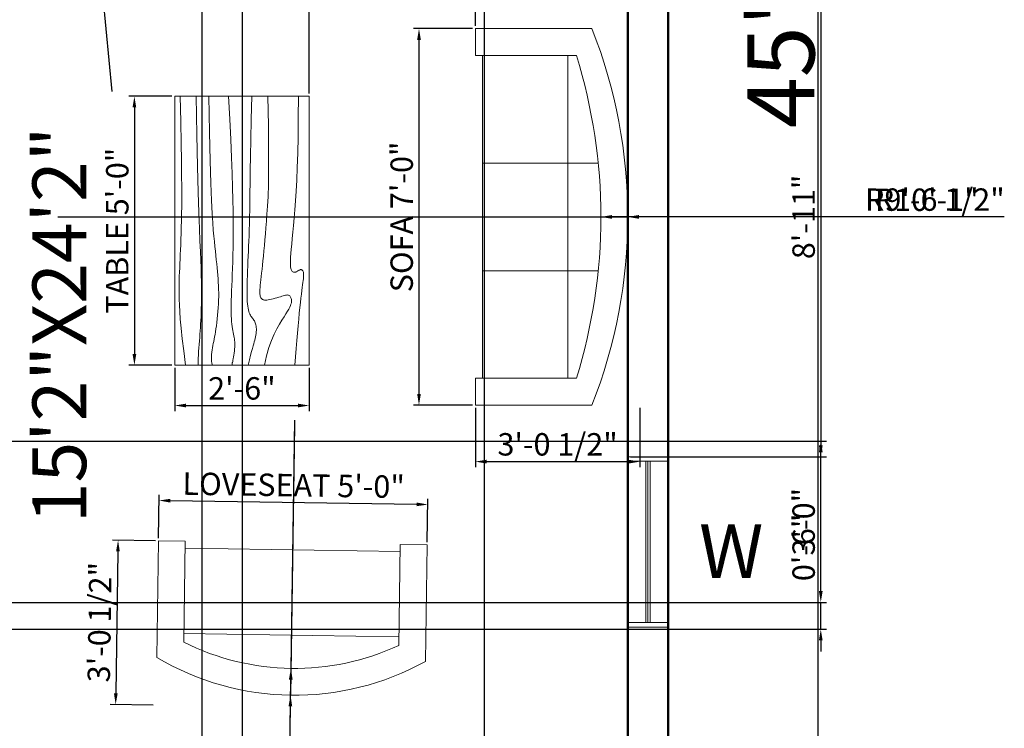
# Model space of a CAD drawing. Units: inches. Extents: x 2050 to 2529, y 1266 to 1968.
# Tile 3 of 5: x 2310 to 2529, y 1427 to 1585. Entities that reach past the tile are written whole.
import ezdxf

# ---------------------------------------------------------------- set-up
doc = ezdxf.new("R2010")
doc.units = ezdxf.units.IN
for name, color, linetype, lineweight in [('A-ANNO-DIMS', 2, 'Continuous', 18), ('A-ANNO-TEXT', 7, 'Continuous', 18), ('A-AREA-IDEN', 7, 'Continuous', 25), ('A-FURN', 8, 'Continuous', 18), ('A-GLAZ', 4, 'Continuous', 18), ('A-WALL', 7, 'Continuous', 50)]:
    doc.layers.add(name, color=color, linetype=linetype, lineweight=lineweight)
doc.styles.get("Standard").update_dxf_attribs({"font": 'arial.ttf'})
doc.dimstyles.new('ISO-25', dxfattribs={"dimtxt": 5, "dimasz": 2.5, "dimexe": 1.25, "dimexo": 0.625, "dimtad": 1, "dimlunit": 3, "dimtxsty": 'Standard', "dimcen": 2.5, "dimadec": 0, "dimazin": 0, "dimtfac": 1, "dimtmove": 0, "dimatfit": 3, "dimfxl": 1, "dimarcsym": 0})

# ---------------------------------------------------------------- blocks, each defined once
blk = doc.blocks.new('*D2')
at = {"layer": 'A-ANNO-DIMS', "color": 0, "lineweight": -2, "transparency": 16777216}
for p, q in [((2454.92, 1844.72), (2488.97, 1844.72)), ((2487.72, 1842.22), (2487.72, 1307.22)), ((2454.92, 1304.72), (2488.97, 1304.72))]:
    blk.add_line(p, q, dxfattribs=at)
at = {"layer": 'A-ANNO-DIMS', "color": 0, "transparency": 16777216}
for points in [[(2487.3, 1842.22), (2488.13, 1842.22), (2487.72, 1844.72)], [(2487.3, 1307.22), (2488.13, 1307.22), (2487.72, 1304.72)]]:
    blk.add_solid(points, dxfattribs=at)
at = {"layer": 'Defpoints', "color": 0, "transparency": 16777216}
for p in [(2454.29, 1844.72), (2454.29, 1304.72), (2487.72, 1304.72)]:
    blk.add_point(p, dxfattribs=at)
at = {"layer": 'A-ANNO-DIMS', "color": 0, "transparency": 16777216, "insert": (2479.46, 1574.72), "char_height": 5, "attachment_point": 5, "rotation": 90}
blk.add_mtext("{\\H3x;45'}", dxfattribs=at)
blk = doc.blocks.new('Table - Rectangular Woodgrain 60 x 30 in.')
for p, q in [((0, 0), (0, -30)), ((60, 0), (0, 0)), ((60, -30), (60, 0)), ((0, -30), (60, -30))]:
    blk.add_line(p, q)
for points in [[(0, -2.4), (4.8155, -2.418), (9.0302, -2.4688), (12.709, -2.5477), (15.9167, -2.65), (18.7181, -2.7711), (21.1781, -2.9063), (23.3616, -3.0508), (25.3333, -3.2), (27.1477, -3.3495), (28.8172, -3.4958), (30.3437, -3.636), (31.7291, -3.7667), (32.9756, -3.8849), (34.0849, -3.9875), (35.059, -4.0714), (35.9, -4.1334), (36.6114, -4.1711), (37.2041, -4.1854), (37.6906, -4.1779), (38.0833, -4.15), (38.3948, -4.1034), (38.6375, -4.0396), (38.8239, -3.9602), (38.9666, -3.8667), (39.0764, -3.7608), (39.1573, -3.6448), (39.2116, -3.521), (39.2416, -3.3917), (39.2498, -3.2593), (39.2385, -3.1261), (39.21, -2.9944), (39.1666, -2.8667), (39.111, -2.7447), (39.0468, -2.6281), (38.978, -2.5163), (38.9083, -2.4083), (38.8418, -2.3035), (38.7823, -2.201), (38.7337, -2.1001), (38.7, -2), (38.6844, -1.9003), (38.6875, -1.8021), (38.7094, -1.707), (38.75, -1.6167), (38.8094, -1.5326), (38.8875, -1.4563), (38.9844, -1.3893), (39.1, -1.3333), (39.2351, -1.2896), (39.3937, -1.2583), (39.5804, -1.2396), (39.8, -1.2333), (40.057, -1.2396), (40.3562, -1.2583), (40.7023, -1.2896), (41.1, -1.3333), (41.5547, -1.3895), (42.0755, -1.4573), (42.6721, -1.5361), (43.3542, -1.625), (44.1316, -1.7233), (45.014, -1.8302), (46.0114, -1.9449), (47.1333, -2.0667), (48.3862, -2.1947), (49.7625, -2.3281), (51.2513, -2.4663), (52.8416, -2.6083), (54.5226, -2.7535), (56.2833, -2.9011), (58.1127, -3.0501), (60, -3.2)], [(0, -9.2), (6.5759, -9.0858), (11.9385, -9.0365), (16.2527, -9.0418), (19.6833, -9.0917), (22.3952, -9.1759), (24.5531, -9.2844), (26.322, -9.4069), (27.8666, -9.5333), (29.3241, -9.6553), (30.7203, -9.7719), (32.0532, -9.8837), (33.3208, -9.9917), (34.5213, -10.0965), (35.6526, -10.199), (36.7128, -10.2999), (37.7, -10.4), (38.6129, -10.4996), (39.4531, -10.5969), (40.223, -10.6895), (40.925, -10.775), (41.5613, -10.8512), (42.1344, -10.9156), (42.6465, -10.966), (43.1, -11), (43.4976, -11.0158), (43.8437, -11.0136), (44.143, -10.9942), (44.4, -10.9583), (44.6195, -10.9069), (44.8062, -10.8406), (44.9648, -10.7603), (45.1, -10.6667), (45.2155, -10.5598), (45.3114, -10.4365), (45.3871, -10.2929), (45.4416, -10.125), (45.4743, -9.929), (45.4844, -9.7011), (45.4709, -9.4371), (45.4333, -9.1333), (45.3716, -8.7883), (45.2896, -8.4104), (45.1919, -8.0107), (45.0833, -7.6), (44.9685, -7.1893), (44.8521, -6.7896), (44.7388, -6.4117), (44.6333, -6.0667), (44.54, -5.7628), (44.4614, -5.4979), (44.4001, -5.2675), (44.3583, -5.0667), (44.3384, -4.8909), (44.3427, -4.7354), (44.3736, -4.5956), (44.4333, -4.4667), (44.5236, -4.3453), (44.6427, -4.2333), (44.7884, -4.1339), (44.9583, -4.05), (45.1501, -3.9849), (45.3614, -3.9417), (45.59, -3.9234), (45.8333, -3.9333), (46.0915, -3.9749), (46.3734, -4.0531), (46.6906, -4.1736), (47.0542, -4.3417), (47.4756, -4.5629), (47.9661, -4.8427), (48.5372, -5.1866), (49.2, -5.6), (49.9676, -6.0844), (50.8594, -6.625), (51.8965, -7.2031), (53.1, -7.8), (54.491, -8.3969), (56.0906, -8.975), (57.9199, -9.5156), (60, -10)], [(0, -12.8), (5.1847, -12.9322), (9.6213, -13.0323), (13.3963, -13.1059), (16.5958, -13.1583), (19.3063, -13.1952), (21.614, -13.2219), (23.6054, -13.2439), (25.3666, -13.2667), (26.9728, -13.2947), (28.4531, -13.3281), (29.8256, -13.3663), (31.1083, -13.4083), (32.3191, -13.4535), (33.476, -13.501), (34.597, -13.5501), (35.7, -13.6), (36.7984, -13.6497), (37.8875, -13.6979), (38.9578, -13.743), (40, -13.7833), (41.0047, -13.8174), (41.9625, -13.8438), (42.864, -13.8607), (43.7, -13.8667), (44.4631, -13.8604), (45.1552, -13.8417), (45.7801, -13.8104), (46.3416, -13.7667), (46.8439, -13.7104), (47.2906, -13.6417), (47.6858, -13.5604), (48.0333, -13.4667), (48.3375, -13.3608), (48.6042, -13.2448), (48.8396, -13.121), (49.05, -12.9917), (49.2417, -12.8593), (49.4208, -12.7261), (49.5937, -12.5944), (49.7667, -12.4667), (49.9452, -12.3451), (50.1323, -12.2313), (50.3303, -12.1268), (50.5416, -12.0333), (50.7686, -11.9524), (51.0135, -11.8854), (51.2788, -11.8341), (51.5666, -11.8), (51.8785, -11.7843), (52.2116, -11.7865), (52.562, -11.8059), (52.926, -11.8417), (53.2998, -11.8931), (53.6795, -11.9594), (54.0614, -12.0397), (54.4416, -12.1333), (54.8223, -12.2401), (55.2293, -12.3625), (55.6942, -12.5037), (56.2489, -12.6667), (56.9251, -12.8547), (57.7545, -13.0708), (58.7689, -13.3182), (60, -13.6)], [(0, -18), (5.124, -17.7273), (9.6609, -17.5057), (13.6705, -17.3303), (17.2125, -17.1958), (20.3467, -17.0973), (23.1328, -17.0297), (25.6307, -16.9878), (27.9, -16.9667), (29.9928, -16.9617), (31.9302, -16.9703), (33.7254, -16.9907), (35.3917, -17.0208), (36.9423, -17.0588), (38.3906, -17.1026), (39.7499, -17.1503), (41.0333, -17.2), (42.2519, -17.2496), (43.4073, -17.2969), (44.4986, -17.3395), (45.525, -17.375), (46.4858, -17.4012), (47.3802, -17.4156), (48.2074, -17.416), (48.9667, -17.4), (49.6583, -17.3662), (50.2872, -17.3167), (50.8595, -17.2547), (51.3812, -17.1833), (51.8584, -17.1057), (52.2971, -17.025), (52.7034, -16.9443), (53.0833, -16.8667), (53.443, -16.7951), (53.789, -16.7313), (54.128, -16.6768), (54.4666, -16.6334), (54.8115, -16.6024), (55.1693, -16.5854), (55.5465, -16.5841), (55.95, -16.6), (56.3828, -16.6337), (56.8346, -16.6823), (57.2915, -16.7418), (57.7396, -16.8084), (58.165, -16.878), (58.5539, -16.9469), (58.8924, -17.0111), (59.1666, -17.0667), (59.3679, -17.1107), (59.5078, -17.1438), (59.6032, -17.1675), (59.6708, -17.1833), (59.7275, -17.193), (59.7901, -17.1979), (59.8753, -17.1998), (60, -17.2)], [(0, -22.4), (8.0098, -22.2501), (14.4094, -22.1011), (19.4168, -21.9535), (23.25, -21.8083), (26.1269, -21.6663), (28.2656, -21.5281), (29.884, -21.3947), (31.2, -21.2667), (32.3967, -21.1448), (33.5172, -21.0292), (34.5697, -20.9198), (35.5625, -20.8167), (36.5037, -20.7198), (37.4015, -20.6292), (38.2642, -20.5448), (39.1, -20.4667), (39.9164, -20.3951), (40.7187, -20.3313), (41.5117, -20.2768), (42.3, -20.2333), (43.0883, -20.2024), (43.8812, -20.1854), (44.6836, -20.1841), (45.5, -20.2), (46.3328, -20.234), (47.1747, -20.2844), (48.0163, -20.3488), (48.8479, -20.425), (49.66, -20.5106), (50.4429, -20.6031), (51.1872, -20.7004), (51.8833, -20.8), (52.5246, -20.8999), (53.1166, -20.9995), (53.6681, -21.0983), (54.1875, -21.1958), (54.6834, -21.2919), (55.1646, -21.3859), (55.6394, -21.4777), (56.1167, -21.5667), (56.6028, -21.6515), (57.0961, -21.7266), (57.5929, -21.7852), (58.0896, -21.8208), (58.5823, -21.8268), (59.0674, -21.7964), (59.5412, -21.723), (60, -21.6)], [(0, -25.2), (8.6355, -25.0504), (15.7026, -24.9031), (21.4049, -24.7606), (25.9458, -24.625), (29.529, -24.4988), (32.3578, -24.3844), (34.6359, -24.284), (36.5667, -24.2), (38.3213, -24.1341), (39.9417, -24.0854), (41.437, -24.0523), (42.8167, -24.0333), (44.0901, -24.0268), (45.2667, -24.0313), (46.3557, -24.0451), (47.3667, -24.0667), (48.309, -24.0947), (49.1928, -24.1287), (50.0284, -24.168), (50.826, -24.2125), (51.5959, -24.2617), (52.3483, -24.3151), (53.0935, -24.3725), (53.8417, -24.4334), (54.6009, -24.497), (55.3699, -24.561), (56.1454, -24.6226), (56.9239, -24.6792), (57.7021, -24.7279), (58.4764, -24.7662), (59.2435, -24.7911), (60, -24.8)], [(0, -28.8), (5.6867, -28.6681), (10.45, -28.5698), (14.407, -28.5012), (17.675, -28.4584), (20.3711, -28.4374), (22.6125, -28.4344), (24.5164, -28.4455), (26.2, -28.4667), (27.762, -28.4947), (29.2276, -28.5281), (30.6033, -28.5663), (31.8958, -28.6084), (33.1118, -28.6535), (34.2578, -28.7011), (35.3405, -28.7501), (36.3666, -28.8), (37.3443, -28.8497), (38.288, -28.8974), (39.2137, -28.9412), (40.1375, -28.9792), (41.0753, -29.0093), (42.0432, -29.0297), (43.0572, -29.0384), (44.1333, -29.0333), (45.2936, -29.0114), (46.5843, -28.9641), (48.0579, -28.8816), (49.7666, -28.7542), (51.7629, -28.5721), (54.0989, -28.3255), (56.8272, -28.0048), (60, -27.6)]]:
    blk.add_lwpolyline(points)
blk = doc.blocks.new('Sofa - Roundback 7 ft.')
for p, q in [((-12.00002, -32.4421), (-12.00003, -6.5971)), ((11.99997, -32.4421), (11.99998, -6.5971)), ((-36.000027, -34), (-36.000027, -11.4696)), ((35.99998, -34), (35.99998, -11.4696)), ((-35.999844, -13.3819), (35.9998, -13.3819)), ((-36.000027, -32.4421), (35.99998, -32.4421))]:
    blk.add_line(p, q)
for points in [[(-36.000027, -34), (-42.000027, -34), (-42.000027, -8)], [(41.99998, -8), (41.99998, -34), (35.99998, -34)]]:
    blk.add_lwpolyline(points)
for centre, radius, start, end in [((0, -114.25), 114.25, 68.43141, 111.5686), ((-0.00001, -127.1968), 121.1968, 72.72033, 107.2797)]:
    blk.add_arc(centre, radius, start, end)
blk = doc.blocks.new('Sofa - Roundback Loveseat 5 ft.')
for p, q in [((0, -32.44198), (0, -5.99998)), ((-24, -33.99998), (-24, -11.46958)), ((24.00004, -33.99998), (24.00004, -11.46958)), ((-23.9998, -13.38178), (23.99986, -13.38178)), ((-24, -32.44198), (24.00004, -32.44198))]:
    blk.add_line(p, q)
for points in [[(-24, -33.99998), (-30, -33.99998), (-30, -7.99998)], [(30.00004, -7.99998), (30.00004, -33.99998), (24.00004, -33.99998)]]:
    blk.add_lwpolyline(points)
for centre, radius, start, end in [((0, -60.24998), 60.24998, 60.13715, 119.8628), ((0, -61.38438), 55.38444, 64.32083, 115.6792)]:
    blk.add_arc(centre, radius, start, end)
blk = doc.blocks.new('WIN-36IN')
for p, q in [((0, 9), (0, 0)), ((1, 9), (1, 0)), ((37, 9), (37, 0)), ((38, 9), (38, 0)), ((1, 5), (37, 5)), ((1, 4.5), (37, 4.5)), ((1, 4), (37, 4))]:
    blk.add_line(p, q)
blk = doc.blocks.new('*D32')
at = {"layer": 'A-ANNO-DIMS', "color": 0, "lineweight": -2, "transparency": 16777216}
for p, q in [((2343.55, 1567.64), (2333.92, 1567.64)), ((2335.17, 1565.14), (2335.17, 1510.14)), ((2343.55, 1507.64), (2333.92, 1507.64))]:
    blk.add_line(p, q, dxfattribs=at)
at = {"layer": 'A-ANNO-DIMS', "color": 0, "transparency": 16777216}
for points in [[(2334.76, 1565.14), (2335.59, 1565.14), (2335.17, 1567.64)], [(2334.76, 1510.14), (2335.59, 1510.14), (2335.17, 1507.64)]]:
    blk.add_solid(points, dxfattribs=at)
at = {"layer": 'Defpoints', "color": 0, "transparency": 16777216}
for p in [(2344.17, 1567.64), (2335.17, 1507.64), (2344.17, 1507.64)]:
    blk.add_point(p, dxfattribs=at)
at = {"layer": 'A-ANNO-DIMS', "color": 0, "transparency": 16777216, "insert": (2332, 1537.64), "char_height": 5, "attachment_point": 5, "rotation": 90}
blk.add_mtext('TABLE 5\'-0"', dxfattribs=at)
blk = doc.blocks.new('*D33')
at = {"layer": 'A-ANNO-DIMS', "color": 0, "lineweight": -2, "transparency": 16777216}
for p, q in [((2344.17, 1507.01), (2344.17, 1497.39)), ((2374.17, 1507.01), (2374.17, 1497.39)), ((2346.67, 1498.64), (2371.67, 1498.64))]:
    blk.add_line(p, q, dxfattribs=at)
at = {"layer": 'A-ANNO-DIMS', "color": 0, "transparency": 16777216}
for points in [[(2346.67, 1499.05), (2346.67, 1498.22), (2344.17, 1498.64)], [(2371.67, 1499.05), (2371.67, 1498.22), (2374.17, 1498.64)]]:
    blk.add_solid(points, dxfattribs=at)
at = {"layer": 'Defpoints', "color": 0, "transparency": 16777216}
for p in [(2344.17, 1507.64), (2374.17, 1507.64), (2374.17, 1498.64)]:
    blk.add_point(p, dxfattribs=at)
at = {"layer": 'A-ANNO-DIMS', "color": 0, "transparency": 16777216, "insert": (2359.17, 1501.81), "char_height": 5, "attachment_point": 5}
blk.add_mtext('2\'-6"', dxfattribs=at)
blk = doc.blocks.new('*D38')
at = {"layer": 'A-ANNO-DIMS', "color": 0, "lineweight": -2, "transparency": 16777216}
for p, q in [((2410.67, 1582.72), (2397.44, 1582.72)), ((2398.69, 1580.22), (2398.69, 1501.22)), ((2410.67, 1498.72), (2397.44, 1498.72))]:
    blk.add_line(p, q, dxfattribs=at)
at = {"layer": 'A-ANNO-DIMS', "color": 0, "transparency": 16777216}
for points in [[(2398.28, 1580.22), (2399.11, 1580.22), (2398.69, 1582.72)], [(2398.28, 1501.22), (2399.11, 1501.22), (2398.69, 1498.72)]]:
    blk.add_solid(points, dxfattribs=at)
at = {"layer": 'Defpoints', "color": 0, "transparency": 16777216}
for p in [(2411.29, 1582.72), (2398.69, 1498.72), (2411.29, 1498.72)]:
    blk.add_point(p, dxfattribs=at)
at = {"layer": 'A-ANNO-DIMS', "color": 0, "transparency": 16777216, "insert": (2395.48, 1540.72), "char_height": 5, "attachment_point": 5, "rotation": 90}
blk.add_mtext('SOFA 7\'-0"', dxfattribs=at)
blk = doc.blocks.new('*D39')
at = {"layer": 'A-ANNO-DIMS', "color": 0, "lineweight": -2, "transparency": 16777216}
for p, q in [((2411.29, 1498.1), (2411.29, 1484.87)), ((2447.96, 1498.1), (2447.96, 1484.87)), ((2413.79, 1486.12), (2445.46, 1486.12))]:
    blk.add_line(p, q, dxfattribs=at)
at = {"layer": 'A-ANNO-DIMS', "color": 0, "transparency": 16777216}
for points in [[(2413.79, 1486.54), (2413.79, 1485.7), (2411.29, 1486.12)], [(2445.46, 1486.54), (2445.46, 1485.7), (2447.96, 1486.12)]]:
    blk.add_solid(points, dxfattribs=at)
at = {"layer": 'Defpoints', "color": 0, "transparency": 16777216}
for p in [(2411.29, 1498.72), (2447.96, 1498.72), (2447.96, 1486.12)]:
    blk.add_point(p, dxfattribs=at)
at = {"layer": 'A-ANNO-DIMS', "color": 0, "transparency": 16777216, "insert": (2429.63, 1489.33), "char_height": 5, "attachment_point": 5}
blk.add_mtext('3\'-0 1/2"', dxfattribs=at)
blk = doc.blocks.new('*D40')
at = {"layer": 'A-ANNO-DIMS', "color": 0, "lineweight": -2, "transparency": 16777216}
for p, q in [((2340.54, 1469.07), (2340.68, 1478.69)), ((2398.16, 1476.58), (2343.17, 1477.4)), ((2400.54, 1468.17), (2400.68, 1477.8))]:
    blk.add_line(p, q, dxfattribs=at)
at = {"layer": 'A-ANNO-DIMS', "color": 0, "transparency": 16777216}
for points in [[(2343.17, 1477.82), (2343.16, 1476.99), (2340.67, 1477.44)], [(2398.17, 1477), (2398.15, 1476.17), (2400.66, 1476.55)]]:
    blk.add_solid(points, dxfattribs=at)
at = {"layer": 'Defpoints', "color": 0, "transparency": 16777216}
for p in [(2340.67, 1477.44), (2340.53, 1468.44), (2400.53, 1467.55)]:
    blk.add_point(p, dxfattribs=at)
at = {"layer": 'A-ANNO-DIMS', "color": 0, "transparency": 16777216, "insert": (2370.71, 1480.21), "char_height": 5, "attachment_point": 5, "rotation": 359.1468}
blk.add_mtext('LOVESEAT 5\'-0"', dxfattribs=at)
blk = doc.blocks.new('*D41')
at = {"layer": 'A-ANNO-DIMS', "color": 0, "lineweight": -2, "transparency": 16777216}
for p, q in [((2339.91, 1468.45), (2330.28, 1468.59)), ((2331.5, 1466.08), (2331.02, 1434.41)), ((2339.36, 1431.79), (2329.74, 1431.93))]:
    blk.add_line(p, q, dxfattribs=at)
at = {"layer": 'A-ANNO-DIMS', "color": 0, "transparency": 16777216}
for points in [[(2331.08, 1466.08), (2331.91, 1466.07), (2331.53, 1468.58)], [(2330.61, 1434.42), (2331.44, 1434.41), (2330.99, 1431.91)]]:
    blk.add_solid(points, dxfattribs=at)
at = {"layer": 'Defpoints', "color": 0, "transparency": 16777216}
for p in [(2340.53, 1468.44), (2330.99, 1431.91), (2339.99, 1431.78)]:
    blk.add_point(p, dxfattribs=at)
at = {"layer": 'A-ANNO-DIMS', "color": 0, "transparency": 16777216, "insert": (2328.05, 1450.29), "char_height": 5, "attachment_point": 5, "rotation": 89.1468}
blk.add_mtext('3\'-0 1/2"', dxfattribs=at)
blk = doc.blocks.new('*D51')
at = {"layer": 'A-ANNO-DIMS', "color": 0, "lineweight": -2, "transparency": 16777216}
for p, q in [((2413.29, 1314.35), (2413.29, 1907.05)), ((2442.79, 1905.8), (2415.79, 1905.8)), ((2445.29, 1314.35), (2445.29, 1907.05))]:
    blk.add_line(p, q, dxfattribs=at)
at = {"layer": 'A-ANNO-DIMS', "color": 0, "transparency": 16777216}
for points in [[(2415.79, 1906.21), (2415.79, 1905.38), (2413.29, 1905.8)], [(2442.79, 1906.21), (2442.79, 1905.38), (2445.29, 1905.8)]]:
    blk.add_solid(points, dxfattribs=at)
at = {"layer": 'Defpoints', "color": 0, "transparency": 16777216}
for p in [(2413.29, 1905.8), (2413.29, 1313.72), (2445.29, 1313.72)]:
    blk.add_point(p, dxfattribs=at)
at = {"layer": 'A-ANNO-DIMS', "color": 0, "transparency": 16777216, "insert": (2429.29, 1908.97), "char_height": 5, "attachment_point": 5}
blk.add_mtext('2\'-8"', dxfattribs=at)
blk = doc.blocks.new('*D52')
at = {"layer": 'A-ANNO-DIMS', "color": 0, "lineweight": -2, "transparency": 16777216}
for p, q in [((2350.29, 1390.35), (2350.29, 1907.05)), ((2352.79, 1905.8), (2356.79, 1905.8)), ((2359.29, 1390.35), (2359.29, 1907.05)), ((2359.29, 1905.8), (2376.34, 1905.8))]:
    blk.add_line(p, q, dxfattribs=at)
at = {"layer": 'A-ANNO-DIMS', "color": 0, "transparency": 16777216}
for points in [[(2352.79, 1906.21), (2352.79, 1905.38), (2350.29, 1905.8)], [(2356.79, 1906.21), (2356.79, 1905.38), (2359.29, 1905.8)]]:
    blk.add_solid(points, dxfattribs=at)
at = {"layer": 'Defpoints', "color": 0, "transparency": 16777216}
for p in [(2359.29, 1905.8), (2350.29, 1389.72), (2359.29, 1389.72)]:
    blk.add_point(p, dxfattribs=at)
at = {"layer": 'A-ANNO-DIMS', "color": 0, "transparency": 16777216, "insert": (2369.07, 1908.97), "char_height": 5, "attachment_point": 5}
blk.add_mtext('0\'-9"', dxfattribs=at)
blk = doc.blocks.new('*D58')
at = {"layer": 'A-ANNO-DIMS', "color": 0, "lineweight": -2, "transparency": 16777216}
for p, q in [((2488.37, 1457.22), (2488.37, 1474.26)), ((2259.92, 1454.72), (2489.62, 1454.72)), ((2488.37, 1448.72), (2488.37, 1454.72)), ((2259.92, 1448.72), (2489.62, 1448.72)), ((2488.37, 1446.22), (2488.37, 1443.72))]:
    blk.add_line(p, q, dxfattribs=at)
at = {"layer": 'A-ANNO-DIMS', "color": 0, "transparency": 16777216}
for points in [[(2487.95, 1457.22), (2488.79, 1457.22), (2488.37, 1454.72)], [(2487.95, 1446.22), (2488.79, 1446.22), (2488.37, 1448.72)]]:
    blk.add_solid(points, dxfattribs=at)
at = {"layer": 'Defpoints', "color": 0, "transparency": 16777216}
for p in [(2259.29, 1454.72), (2488.37, 1454.72), (2259.29, 1448.72)]:
    blk.add_point(p, dxfattribs=at)
at = {"layer": 'A-ANNO-DIMS', "color": 0, "transparency": 16777216, "insert": (2485.19, 1466.99), "char_height": 5, "attachment_point": 5, "rotation": 90}
blk.add_mtext('0\'-6"', dxfattribs=at)
blk = doc.blocks.new('*D59')
at = {"layer": 'A-ANNO-DIMS', "color": 0, "lineweight": -2, "transparency": 16777216}
for p, q in [((2259.92, 1490.72), (2489.62, 1490.72)), ((2488.37, 1457.22), (2488.37, 1488.22)), ((2259.92, 1454.72), (2489.62, 1454.72))]:
    blk.add_line(p, q, dxfattribs=at)
at = {"layer": 'A-ANNO-DIMS', "color": 0, "transparency": 16777216}
for points in [[(2487.95, 1488.22), (2488.79, 1488.22), (2488.37, 1490.72)], [(2487.95, 1457.22), (2488.79, 1457.22), (2488.37, 1454.72)]]:
    blk.add_solid(points, dxfattribs=at)
at = {"layer": 'Defpoints', "color": 0, "transparency": 16777216}
for p in [(2259.29, 1490.72), (2488.37, 1490.72), (2259.29, 1454.72)]:
    blk.add_point(p, dxfattribs=at)
at = {"layer": 'A-ANNO-DIMS', "color": 0, "transparency": 16777216, "insert": (2485.19, 1472.72), "char_height": 5, "attachment_point": 5, "rotation": 90}
blk.add_mtext('3\'-0"', dxfattribs=at)
blk = doc.blocks.new('*D72')
at = {"layer": 'A-ANNO-DIMS', "color": 0, "lineweight": -2, "transparency": 16777216}
for p, q in [((2445.92, 1594.22), (2489.62, 1594.22)), ((2488.37, 1591.72), (2488.37, 1489.72)), ((2445.92, 1487.22), (2489.62, 1487.22))]:
    blk.add_line(p, q, dxfattribs=at)
at = {"layer": 'A-ANNO-DIMS', "color": 0, "transparency": 16777216}
for points in [[(2487.95, 1591.72), (2488.79, 1591.72), (2488.37, 1594.22)], [(2487.95, 1489.72), (2488.79, 1489.72), (2488.37, 1487.22)]]:
    blk.add_solid(points, dxfattribs=at)
at = {"layer": 'Defpoints', "color": 0, "transparency": 16777216}
for p in [(2445.29, 1594.22), (2445.29, 1487.22), (2488.37, 1487.22)]:
    blk.add_point(p, dxfattribs=at)
at = {"layer": 'A-ANNO-DIMS', "color": 0, "transparency": 16777216, "insert": (2485.19, 1540.72), "char_height": 5, "attachment_point": 5, "rotation": 90}
blk.add_mtext('8\'-11"', dxfattribs=at)
blk = doc.blocks.new('*D79')
at = {"layer": 'A-ANNO-DIMS', "color": 0, "lineweight": -2, "transparency": 16777216}
for p, q in [((2374.17, 1568.26), (2374.17, 1907.05)), ((2376.67, 1905.8), (2408.79, 1905.8)), ((2411.29, 1583.35), (2411.29, 1907.05))]:
    blk.add_line(p, q, dxfattribs=at)
at = {"layer": 'A-ANNO-DIMS', "color": 0, "transparency": 16777216}
for points in [[(2376.67, 1906.21), (2376.67, 1905.38), (2374.17, 1905.8)], [(2408.79, 1906.21), (2408.79, 1905.38), (2411.29, 1905.8)]]:
    blk.add_solid(points, dxfattribs=at)
at = {"layer": 'Defpoints', "color": 0, "transparency": 16777216}
for p in [(2411.29, 1905.8), (2411.29, 1582.72), (2374.17, 1567.64)]:
    blk.add_point(p, dxfattribs=at)
at = {"layer": 'A-ANNO-DIMS', "color": 0, "transparency": 16777216, "insert": (2392.73, 1908.98), "char_height": 5, "attachment_point": 5}
blk.add_mtext('3\'-1"', dxfattribs=at)
blk = doc.blocks.new('*D80')
at = {"layer": 'A-ANNO-DIMS', "color": 0, "lineweight": -2, "transparency": 16777216}
for p, q in [((2318.1, 1540.72), (2439.29, 1540.72)), ((2523.62, 1540.72), (2441.79, 1540.72))]:
    blk.add_line(p, q, dxfattribs=at)
at = {"layer": 'A-ANNO-DIMS', "color": 0, "transparency": 16777216}
blk.add_solid([(2441.79, 1541.14), (2441.79, 1540.3), (2439.29, 1540.72)], dxfattribs=at)
at = {"layer": 'Defpoints', "color": 0, "transparency": 16777216}
for p in [(2318.1, 1540.72), (2439.29, 1540.72)]:
    blk.add_point(p, dxfattribs=at)
at = {"layer": 'A-ANNO-DIMS', "color": 0, "transparency": 16777216, "insert": (2512.01, 1543.9), "char_height": 5, "attachment_point": 5, "rotation": 359.9998}
blk.add_mtext('R10\'-1"', dxfattribs=at)
blk = doc.blocks.new('*D81')
at = {"layer": 'A-ANNO-DIMS', "color": 0, "lineweight": -2, "transparency": 16777216}
for p, q in [((2331.04, 1540.72), (2445.29, 1540.72)), ((2529.33, 1540.72), (2447.79, 1540.72))]:
    blk.add_line(p, q, dxfattribs=at)
at = {"layer": 'A-ANNO-DIMS', "color": 0, "transparency": 16777216}
blk.add_solid([(2447.79, 1541.14), (2447.79, 1540.3), (2445.29, 1540.72)], dxfattribs=at)
at = {"layer": 'Defpoints', "color": 0, "transparency": 16777216}
for p in [(2331.04, 1540.72), (2445.29, 1540.72)]:
    blk.add_point(p, dxfattribs=at)
at = {"layer": 'A-ANNO-DIMS', "color": 0, "transparency": 16777216, "insert": (2513.84, 1543.93), "char_height": 5, "attachment_point": 5, "rotation": 359.9998}
blk.add_mtext('R9\'-6 1/2"', dxfattribs=at)
blk = doc.blocks.new('*D82')
at = {"layer": 'A-ANNO-DIMS', "color": 0, "lineweight": -2, "transparency": 16777216}
for p, q in [((2318.3, 1691.92), (2323.8, 1635.17)), ((2330.24, 1568.73), (2324.04, 1632.68))]:
    blk.add_line(p, q, dxfattribs=at)
at = {"layer": 'A-ANNO-DIMS', "color": 0, "transparency": 16777216}
blk.add_solid([(2324.21, 1635.21), (2323.38, 1635.13), (2324.04, 1632.68)], dxfattribs=at)
at = {"layer": 'Defpoints', "color": 0, "transparency": 16777216}
for p in [(2324.04, 1632.68), (2330.24, 1568.73)]:
    blk.add_point(p, dxfattribs=at)
at = {"layer": 'A-ANNO-DIMS', "color": 0, "transparency": 16777216, "insert": (2323.52, 1671.36), "char_height": 5, "attachment_point": 5, "rotation": 275.5377}
blk.add_mtext('4X R5\'-4 1/2"', dxfattribs=at)
blk = doc.blocks.new('*D83')
at = {"layer": 'A-ANNO-DIMS', "color": 0, "lineweight": -2, "transparency": 16777216}
for p, q in [((2370.92, 1494.24), (2370.02, 1434)), ((2369.34, 1388.19), (2369.99, 1431.5))]:
    blk.add_line(p, q, dxfattribs=at)
at = {"layer": 'A-ANNO-DIMS', "color": 0, "transparency": 16777216}
blk.add_solid([(2369.57, 1431.51), (2370.4, 1431.49), (2370.02, 1434)], dxfattribs=at)
at = {"layer": 'Defpoints', "color": 0, "transparency": 16777216}
for p in [(2370.92, 1494.24), (2370.02, 1434)]:
    blk.add_point(p, dxfattribs=at)
at = {"layer": 'A-ANNO-DIMS', "color": 0, "transparency": 16777216, "insert": (2366.31, 1397.9), "char_height": 5, "attachment_point": 5, "rotation": 89.147}
blk.add_mtext('R5\'-0"', dxfattribs=at)
blk = doc.blocks.new('*D84')
at = {"layer": 'A-ANNO-DIMS', "color": 0, "lineweight": -2, "transparency": 16777216}
for p, q in [((2370.94, 1495.38), (2370.11, 1440)), ((2369.39, 1391.28), (2370.07, 1437.5))]:
    blk.add_line(p, q, dxfattribs=at)
at = {"layer": 'A-ANNO-DIMS', "color": 0, "transparency": 16777216}
blk.add_solid([(2369.66, 1437.5), (2370.49, 1437.49), (2370.11, 1440)], dxfattribs=at)
at = {"layer": 'Defpoints', "color": 0, "transparency": 16777216}
for p in [(2370.94, 1495.38), (2370.11, 1440)]:
    blk.add_point(p, dxfattribs=at)
at = {"layer": 'A-ANNO-DIMS', "color": 0, "transparency": 16777216, "insert": (2366.41, 1406.82), "char_height": 5, "attachment_point": 5, "rotation": 89.1467}
blk.add_mtext('R4\'-7 1/2"', dxfattribs=at)

msp = doc.modelspace()

# ---------------------------------------------------------------- linework, layer by layer
at = {"layer": 'A-WALL'}
for p, q in [((2454.295, 1844.72), (2454.295, 1304.72)), ((2445.295, 1685.72), (2445.295, 1395.72))]:
    msp.add_line(p, q, dxfattribs=at)

# ---------------------------------------------------------------- block references
at = {"layer": 'A-FURN'}
for name, p, rotation in [('Sofa - Roundback 7 ft.', (2445.295, 1540.72), 270), ('Table - Rectangular Woodgrain 60 x 30 in.', (2374.175, 1567.637), 270), ('Sofa - Roundback Loveseat 5 ft.', (2370.023, 1433.999), 179.1468455893285)]:
    msp.add_blockref(name, p, dxfattribs=dict(at, rotation=rotation))
at = {"layer": 'A-GLAZ', "rotation": 269.9999999999999}
msp.add_blockref('WIN-36IN', (2445.294, 1487.22), dxfattribs=at)

# ---------------------------------------------------------------- texts
at = {"layer": 'A-ANNO-TEXT', "insert": (2461.189, 1472.151), "char_height": 12, "attachment_point": 1}
msp.add_mtext_dynamic_manual_height_columns('W', width=471.52273, gutter_width=12.5, heights=[28.462], dxfattribs=at)
at = {"layer": 'A-AREA-IDEN', "insert": (2292.409, 1472.375), "char_height": 12, "attachment_point": 1, "rotation": 90}
msp.add_mtext_dynamic_manual_height_columns('LIVING HALL\\P15\'2"X24\'2"', width=649.2389, gutter_width=12.5, heights=[75.088], dxfattribs=at)

# ---------------------------------------------------------------- dimensions: what is measured, and where the dimension line sits
at = {"layer": 'A-ANNO-DIMS'}
for base, p1, p2, picture, middle in [((2359.295, 1905.795), (2350.295, 1389.72), (2359.295, 1389.72), '*D52', (2369.065, 1908.973)), ((2411.295, 1905.795), (2374.175, 1567.637), (2411.295, 1582.72), '*D79', (2392.735, 1908.975)), ((2413.295, 1905.795), (2445.295, 1313.72), (2413.295, 1313.72), '*D51', (2429.295, 1908.973)), ((2374.175, 1498.637), (2344.175, 1507.637), (2374.175, 1507.637), '*D33', (2359.175, 1501.815)), ((2447.961, 1486.12), (2411.295, 1498.72), (2447.961, 1498.72), '*D39', (2429.628, 1489.332))]:
    dim = msp.add_linear_dim(base=base, p1=p1, p2=p2, dimstyle='ISO-25', override={"dimdec": 1, "dimlfac": 1, "dimrnd": 0, "dimzin": 1, "dimdsep": 46, "dimlunit": 4, "dimfrac": 2}, dxfattribs=at)
    dim.commit()
    dim.dimension.update_dxf_attribs({"geometry": picture, "text_midpoint": middle})
for base, p1, p2, angle, text, override, picture, middle in [((2487.716, 1304.72), (2454.295, 1844.72), (2454.295, 1304.72), 90, '{\\H3x;<>}', {"dimclrd": 0, "dimclre": 0, "dimclrt": 0}, '*D2', (2479.463, 1574.72)), ((2398.695, 1498.72), (2411.295, 1582.72), (2411.295, 1498.72), 270, 'SOFA <>', {"dimdec": 1, "dimlfac": 1, "dimrnd": 0, "dimzin": 1, "dimdsep": 46, "dimlunit": 4, "dimfrac": 2}, '*D38', (2395.483, 1540.72)), ((2335.175, 1507.637), (2344.175, 1567.637), (2344.175, 1507.637), 270, 'TABLE <>', {"dimdec": 1, "dimlfac": 1, "dimrnd": 0, "dimzin": 1, "dimdsep": 46, "dimlunit": 4, "dimfrac": 2}, '*D32', (2331.997, 1537.637)), ((2340.666, 1477.44), (2400.526, 1467.548), (2340.532, 1468.441), 179.14685, 'LOVESEAT <>', {"dimdec": 1, "dimlfac": 1, "dimrnd": 0, "dimzin": 1, "dimdsep": 46, "dimlunit": 4, "dimfrac": 2}, '*D40', (2370.711, 1480.205))]:
    dim = msp.add_linear_dim(base=base, p1=p1, p2=p2, angle=angle, text=text, dimstyle='ISO-25', override=override, dxfattribs=at)
    dim.commit()
    dim.dimension.update_dxf_attribs({"geometry": picture, "text_midpoint": middle})
dim = msp.add_radius_dim(center=(2330.24017, 1568.73218), mpoint=(2324.03997, 1632.68232), text='4X <>', dimstyle='ISO-25', override={"dimdec": 1, "dimlfac": 1, "dimrnd": 0, "dimzin": 1, "dimdsep": 46, "dimlunit": 4, "dimfrac": 2}, dxfattribs=at)
dim.commit()
dim.dimension.update_dxf_attribs({"geometry": '*D82', "text_midpoint": (2320.31985, 1671.0524), "dimtype": 164})
for base, p1, p2, angle, picture, middle in [((2488.37, 1487.22), (2445.295, 1594.22), (2445.295, 1487.22), 90, '*D72', (2485.192, 1540.72)), ((2488.37, 1490.72), (2259.295, 1454.72), (2259.295, 1490.72), 90, '*D59', (2485.19, 1472.72)), ((2488.37, 1454.72), (2259.295, 1448.72), (2259.295, 1454.72), 90, '*D58', (2485.192, 1466.991)), ((2330.987, 1431.913), (2340.532, 1468.441), (2339.986, 1431.779), 269.14685, '*D41', (2328.049, 1450.292))]:
    dim = msp.add_linear_dim(base=base, p1=p1, p2=p2, angle=angle, dimstyle='ISO-25', override={"dimdec": 1, "dimlfac": 1, "dimrnd": 0, "dimzin": 1, "dimdsep": 46, "dimlunit": 4, "dimfrac": 2}, dxfattribs=at)
    dim.commit()
    dim.dimension.update_dxf_attribs({"geometry": picture, "text_midpoint": middle})
for center, mpoint, picture, middle in [((2331.044714, 1540.720434), (2445.294714, 1540.72), '*D81', (2513.844714, 1540.7197396)), ((2318.098, 1540.72), (2439.295, 1540.72), '*D80', (2512.013, 1540.72)), ((2370.937, 1495.376), (2370.112, 1439.998), '*D84', (2369.617, 1406.771)), ((2370.92, 1494.242), (2370.023, 1433.999), '*D83', (2369.485, 1397.853))]:
    dim = msp.add_radius_dim(center=center, mpoint=mpoint, dimstyle='ISO-25', override={"dimdec": 1, "dimlfac": 1, "dimrnd": 0, "dimzin": 1, "dimdsep": 46, "dimlunit": 4, "dimfrac": 2}, dxfattribs=at)
    dim.commit()
    dim.dimension.update_dxf_attribs({"geometry": picture, "text_midpoint": middle, "dimtype": 164})

doc.saveas('drawing.dxf')
